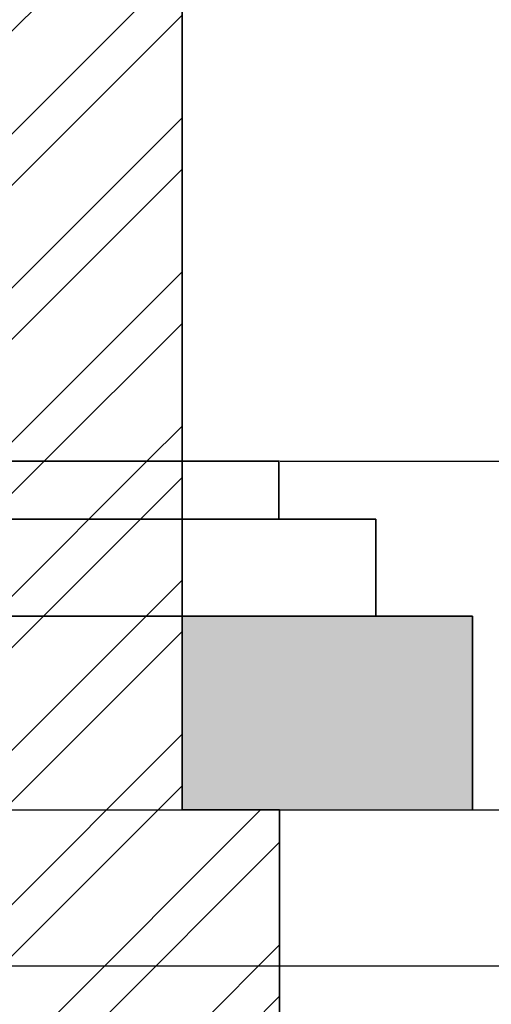
# Model space of a CAD drawing. Units: inches. Extents: x -301 to 715, y -607 to 364.
# Tile 35 of 141: x 135 to 159, y -492 to -441. Entities that reach past the tile are written whole.
import ezdxf

# ---------------------------------------------------------------- set-up
doc = ezdxf.new("R2010")
doc.units = ezdxf.units.IN
doc.header["$MEASUREMENT"] = 0
for name, color, linetype, lineweight in [('A-ANNO-DIMS', 2, 'Continuous', 18), ('A-GRND', 7, 'Continuous', 25), ('A-SECT', 1, 'Continuous', 35), ('A-SECT-PATT', 8, 'Continuous', 13), ('S-FNDN', 2, 'Continuous', 35)]:
    doc.layers.add(name, color=color, linetype=linetype, lineweight=lineweight)
doc.styles.get("Standard").update_dxf_attribs({"font": 'arial.ttf'})
doc.dimstyles.get("Standard").update_dxf_attribs({"dimtxt": 0.18, "dimasz": 0.18, "dimexe": 0.18, "dimexo": 0.0625, "dimgap": 0.09, "dimtad": 0, "dimtih": 1, "dimtoh": 1, "dimdec": 1, "dimzin": 0, "dimdsep": 46, "dimlunit": 4, "dimtxsty": 'Standard', "dimcen": 0.09, "dimclrd": 3, "dimclre": 4, "dimclrt": 6, "dimadec": 0, "dimazin": 0, "dimtfac": 1, "dimtdec": 1, "dimtofl": 0, "dimtmove": 0, "dimatfit": 3, "dimfxl": 1, "dimtfill": 2, "dimtfillclr": 51, "dimtolj": 1, "dimtzin": 0, "dimarcsym": 0})
pattern_1 = [(45, (10.321, 33.8764), (-3.977476, 3.977476), []), (45, (12.973, 33.8764), (-3.977476, 3.977476), [])]

# ---------------------------------------------------------------- blocks, each defined once
blk = doc.blocks.new('*D76')
at = {"layer": 'A-ANNO-DIMS', "color": 0, "lineweight": -2, "transparency": 16777216}
for p, q in [((158.28, -324.519), (162.311, -324.519)), ((162.131, -329.519), (162.131, -400.354)), ((162.131, -476.477), (162.131, -405.643)), ((158.28, -481.477), (162.311, -481.477))]:
    blk.add_line(p, q, dxfattribs=at)
at = {"layer": 'A-ANNO-DIMS', "color": 0, "transparency": 16777216}
for points in [[(161.297, -329.519), (162.964, -329.519), (162.131, -324.519)], [(161.297, -476.477), (162.964, -476.477), (162.131, -481.477)]]:
    blk.add_solid(points, dxfattribs=at)
at = {"layer": 'Defpoints', "color": 0, "transparency": 16777216}
for p in [(158.218, -324.519), (162.131, -324.519), (158.218, -481.477)]:
    blk.add_point(p, dxfattribs=at)
at = {"layer": 'A-ANNO-DIMS', "color": 0, "transparency": 16777216, "insert": (162.131, -402.998), "char_height": 5, "attachment_point": 5, "bg_fill": 1, "box_fill_scale": 1.25, "bg_fill_color": 51, "bg_fill_transparency": 0}
blk.add_mtext('\\A1;13\'-1"', dxfattribs=at)
blk = doc.blocks.new('*D80')
at = {"layer": 'A-ANNO-DIMS', "color": 0, "lineweight": -2, "transparency": 16777216}
for p, q in [((176.814, -481.477), (176.814, -476.477)), ((176.814, -476.477), (181.814, -476.477)), ((153.318, -481.477), (176.994, -481.477)), ((176.814, -488.477), (176.814, -486.477)), ((153.318, -493.477), (176.994, -493.477))]:
    blk.add_line(p, q, dxfattribs=at)
at = {"layer": 'A-ANNO-DIMS', "color": 0, "transparency": 16777216}
for points in [[(175.981, -486.477), (177.648, -486.477), (176.814, -481.477)], [(175.981, -488.477), (177.648, -488.477), (176.814, -493.477)]]:
    blk.add_solid(points, dxfattribs=at)
at = {"layer": 'Defpoints', "color": 0, "transparency": 16777216}
for p in [(153.255, -481.477), (176.814, -481.477), (153.255, -493.477)]:
    blk.add_point(p, dxfattribs=at)
at = {"layer": 'A-ANNO-DIMS', "color": 0, "transparency": 16777216, "insert": (183.969, -476.477), "char_height": 5, "attachment_point": 5, "bg_fill": 1, "box_fill_scale": 1.25, "bg_fill_color": 51, "bg_fill_transparency": 0}
blk.add_mtext("\\A1;1'", dxfattribs=at)
blk = doc.blocks.new('*D81')
at = {"layer": 'A-ANNO-DIMS', "color": 0, "lineweight": -2, "transparency": 16777216}
for p, q in [((155.28, -385.477), (177.024, -385.477)), ((176.844, -390.477), (176.844, -430.835)), ((176.844, -476.477), (176.844, -436.12)), ((158.28, -481.477), (177.024, -481.477))]:
    blk.add_line(p, q, dxfattribs=at)
at = {"layer": 'A-ANNO-DIMS', "color": 0, "transparency": 16777216}
for points in [[(176.011, -390.477), (177.678, -390.477), (176.844, -385.477)], [(176.011, -476.477), (177.678, -476.477), (176.844, -481.477)]]:
    blk.add_solid(points, dxfattribs=at)
at = {"layer": 'Defpoints', "color": 0, "transparency": 16777216}
for p in [(155.218, -385.477), (158.218, -481.477), (176.844, -481.477)]:
    blk.add_point(p, dxfattribs=at)
at = {"layer": 'A-ANNO-DIMS', "color": 0, "transparency": 16777216, "insert": (176.844, -433.477), "char_height": 5, "attachment_point": 5, "bg_fill": 1, "box_fill_scale": 1.25, "bg_fill_color": 51, "bg_fill_transparency": 0}
blk.add_mtext("\\A1;8'", dxfattribs=at)
blk = doc.blocks.new('*D176')
at = {"layer": 'A-ANNO-DIMS', "color": 4, "lineweight": -2, "transparency": 16777216}
for p, q in [((148.28, -324.477), (215.605, -324.477)), ((-15.22, -540.477), (215.605, -540.477))]:
    blk.add_line(p, q, dxfattribs=at)
at = {"layer": 'A-ANNO-DIMS', "color": 3, "lineweight": -2, "transparency": 16777216}
for p, q in [((215.425, -324.657), (215.425, -432.296)), ((215.425, -540.297), (215.425, -432.659))]:
    blk.add_line(p, q, dxfattribs=at)
at = {"layer": 'A-ANNO-DIMS', "color": 3, "transparency": 16777216}
for points in [[(215.395, -324.657), (215.455, -324.657), (215.425, -324.477)], [(215.395, -540.297), (215.455, -540.297), (215.425, -540.477)]]:
    blk.add_solid(points, dxfattribs=at)
at = {"layer": 'Defpoints', "color": 0, "transparency": 16777216}
for p in [(148.218, -324.477), (-15.282, -540.477), (215.425, -540.477)]:
    blk.add_point(p, dxfattribs=at)
at = {"layer": 'A-ANNO-DIMS', "color": 6, "transparency": 16777216, "insert": (215.425, -432.477), "char_height": 0.18, "attachment_point": 5, "bg_fill": 1, "box_fill_scale": 1.25, "bg_fill_color": 51, "bg_fill_transparency": 0}
blk.add_mtext('\\A1;18\'-0"', dxfattribs=at)
blk = doc.blocks.new('*D188')
at = {"layer": 'A-ANNO-DIMS', "color": 4, "lineweight": -2, "transparency": 16777216}
for p, q in [((148.28, -463.477), (215.605, -463.477)), ((158.28, -481.477), (215.605, -481.477))]:
    blk.add_line(p, q, dxfattribs=at)
at = {"layer": 'A-ANNO-DIMS', "color": 3, "lineweight": -2, "transparency": 16777216}
for p, q in [((215.425, -463.657), (215.425, -472.296)), ((215.425, -481.297), (215.425, -472.659))]:
    blk.add_line(p, q, dxfattribs=at)
at = {"layer": 'A-ANNO-DIMS', "color": 3, "transparency": 16777216}
for points in [[(215.395, -463.657), (215.455, -463.657), (215.425, -463.477)], [(215.395, -481.297), (215.455, -481.297), (215.425, -481.477)]]:
    blk.add_solid(points, dxfattribs=at)
at = {"layer": 'Defpoints', "color": 0, "transparency": 16777216}
for p in [(148.218, -463.477), (215.425, -463.477), (158.218, -481.477)]:
    blk.add_point(p, dxfattribs=at)
at = {"layer": 'A-ANNO-DIMS', "color": 6, "transparency": 16777216, "insert": (215.425, -472.477), "char_height": 0.18, "attachment_point": 5, "bg_fill": 1, "box_fill_scale": 1.25, "bg_fill_color": 51, "bg_fill_transparency": 0}
blk.add_mtext('\\A1;1\'-6"', dxfattribs=at)
blk = doc.blocks.new('*D200')
at = {"layer": 'A-ANNO-DIMS', "color": 4, "lineweight": -2, "transparency": 16777216}
for p, q in [((412.955, -393.552), (121.926, -393.552)), ((412.955, -489.552), (121.926, -489.552))]:
    blk.add_line(p, q, dxfattribs=at)
at = {"layer": 'A-ANNO-DIMS', "color": 3, "lineweight": -2, "transparency": 16777216}
for p, q in [((122.106, -393.732), (122.106, -441.371)), ((122.106, -489.372), (122.106, -441.734))]:
    blk.add_line(p, q, dxfattribs=at)
at = {"layer": 'A-ANNO-DIMS', "color": 3, "transparency": 16777216}
for points in [[(122.076, -393.732), (122.136, -393.732), (122.106, -393.552)], [(122.076, -489.372), (122.136, -489.372), (122.106, -489.552)]]:
    blk.add_solid(points, dxfattribs=at)
at = {"layer": 'Defpoints', "color": 0, "transparency": 16777216}
for p in [(122.106, -393.552), (413.018, -393.552), (413.018, -489.552)]:
    blk.add_point(p, dxfattribs=at)
at = {"layer": 'A-ANNO-DIMS', "color": 6, "transparency": 16777216, "insert": (122.106, -441.552), "char_height": 0.18, "attachment_point": 5, "bg_fill": 1, "box_fill_scale": 1.25, "bg_fill_color": 51, "bg_fill_transparency": 0}
blk.add_mtext('\\A1;8\'-0"', dxfattribs=at)

msp = doc.modelspace()

# ---------------------------------------------------------------- hatches: boundary and pattern name
at = {"layer": 'A-SECT-PATT'}
h = msp.add_hatch(dxfattribs=at)
h.set_pattern_fill('ANSI32', color=256, scale=15)
h.set_pattern_definition(pattern_1)
h.paths.add_polyline_path([(-185.282, -324.477), (-199.282, -324.477), (-199.282, -329.477), (-194.282, -329.477), (-194.282, -353.477), (-185.282, -353.477)])
h.paths.add_polyline_path([(-185.282, -361.477), (-193.904, -361.477), (-193.982, -377.537), (-185.282, -377.537)])
h.paths.add_polyline_path([(143.218, -329.477), (148.218, -329.477), (148.218, -324.477), (134.255, -324.477), (134.255, -353.477), (143.218, -353.477)])
h.paths.add_polyline_path([(143.218, -361.477), (134.255, -361.477), (134.255, -377.477), (143.218, -377.477)])
h.paths.add_polyline_path([(-185.282, -439.477), (-194.282, -439.477), (-194.282, -463.477), (-185.282, -463.477)])
h.paths.add_polyline_path([(-185.282, -471.477), (-194.282, -471.477), (-194.282, -481.477), (-185.282, -481.477)])
h.paths.add_polyline_path([(-185.282, -463.477), (-194.282, -463.477), (-194.282, -466.477), (-185.282, -466.477)])
h.paths.add_polyline_path([(-185.282, -466.477), (-194.282, -466.477), (-194.282, -471.477), (-185.282, -471.477)])
h.paths.add_polyline_path([(-180.282, -481.477), (-185.282, -481.477), (-194.282, -481.477), (-199.282, -481.477), (-199.282, -493.477), (-180.282, -493.477)])
h.paths.add_polyline_path([(-175.282, -493.477), (-180.282, -493.477), (-199.282, -493.477), (-204.282, -493.477), (-204.282, -511.477), (-175.282, -511.477)])
h.paths.add_polyline_path([(-170.282, -511.477), (-175.282, -511.477), (-204.282, -511.477), (-209.282, -511.477), (-209.282, -535.477), (-170.282, -535.477)])
h.paths.add_polyline_path([(-35.282, -463.477), (-41.282, -463.477), (-41.282, -466.477), (-35.282, -466.477)])
h.paths.add_polyline_path([(-35.282, -466.477), (-41.282, -466.477), (-41.282, -471.477), (-35.282, -471.477)])
h.paths.add_polyline_path([(-35.282, -471.477), (-41.282, -471.477), (-41.282, -481.477), (-35.282, -481.477)])
h.paths.add_polyline_path([(-30.282, -481.477), (-46.282, -481.477), (-46.282, -493.477), (-30.282, -493.477)])
h.paths.add_polyline_path([(-25.282, -493.477), (-30.282, -493.477), (-46.282, -493.477), (-51.282, -493.477), (-51.282, -511.477), (-25.282, -511.477)])
h.paths.add_polyline_path([(-20.282, -511.477), (-25.282, -511.477), (-51.282, -511.477), (-56.282, -511.477), (-56.282, -535.477), (-20.282, -535.477)])
h.paths.add_polyline_path([(143.218, -463.477), (134.255, -463.477), (134.255, -466.477), (143.218, -466.477)])
h.paths.add_polyline_path([(143.218, -466.477), (134.255, -466.477), (134.255, -471.477), (143.218, -471.477)])
h.paths.add_polyline_path([(143.218, -471.477), (134.255, -471.477), (134.255, -481.477), (143.218, -481.477)])
h.paths.add_polyline_path([(148.255, -481.477), (143.255, -481.477), (134.255, -481.477), (129.255, -481.477), (129.255, -493.477), (148.255, -493.477)])
h.paths.add_polyline_path([(153.255, -493.477), (148.255, -493.477), (129.255, -493.477), (124.255, -493.477), (124.255, -511.477), (153.255, -511.477)])
h.paths.add_polyline_path([(158.255, -511.477), (153.255, -511.477), (124.255, -511.477), (119.255, -511.477), (119.255, -535.477), (158.255, -535.477)])
h = msp.add_hatch(dxfattribs=at)
h.set_pattern_fill('AR-CONC', color=256, scale=0.5)
h.set_pattern_definition([(50, (10.3213, 33.8764), (3.586301, -0.31376), [0.375, -4.125]), (355, (10.3213, 33.8764), (-0.693757, 3.76096), [0.3, -3.3]), (100.45144, (10.62, 33.8502), (2.892544, 3.4472), [0.3187, -3.50571]), (46.1842, (10.3213, 34.8764), (5.336207, -0.827596), [0.5625, -6.1875]), (96.6356, (10.766, 34.8074), (4.67331, 4.870593), [0.47805, -5.25857]), (351.1842, (10.321, 34.8764), (4.67331, 4.870593), [0.45, -4.95]), (21, (10.8213, 34.6264), (2.984535, -2.013094), [0.375, -4.125]), (326, (10.8213, 34.6264), (1.216577, 3.62575), [0.3, -3.3]), (71.45144, (11.07, 34.4586), (4.201112, 1.612656), [0.3187, -3.50571]), (37.5, (10.3213, 33.8764), (0.0607993, 1.6644693), [0, -3.26, 0, -3.35, 0, -3.3125]), (7.5, (10.3213, 33.8764), (1.3153477, 1.9720586), [0, -1.91, 0, -3.185, 0, -1.2625]), (327.5, (9.2063, 33.8764), (2.6691122, -0.1127744), [0, -1.25, 0, -3.9, 0, -5.175]), (317.5, (8.7063, 33.8764), (2.915931, 0.500525), [0, -1.625, 0, -2.59, 0, -3.675])])
h.paths.add_polyline_path([(-56.282, -535.477), (-61.282, -535.477), (-61.282, -540.477), (-15.282, -540.477), (-15.282, -535.477), (-20.282, -535.477)])
h.paths.add_polyline_path([(119.255, -535.477), (114.255, -535.477), (114.255, -540.477), (163.255, -540.477), (163.255, -535.477), (158.255, -535.477)])
h.paths.add_polyline_path([(-206.282, -471.477), (-209.282, -471.477), (-209.282, -481.477), (-206.282, -481.477), (-194.282, -481.477), (-194.282, -471.477)])
h.paths.add_polyline_path([(-41.282, -481.477), (-41.282, -471.477), (-185.282, -471.477), (-185.282, -481.477), (-180.282, -481.477)])
h.paths.add_polyline_path([(134.255, -481.477), (134.255, -471.477), (-35.282, -471.477), (-35.282, -481.477), (-30.282, -481.477)])
h.paths.add_polyline_path([(155.218, -481.477), (158.218, -481.477), (158.218, -471.477), (153.218, -471.477), (143.218, -471.477), (143.218, -481.477), (148.255, -481.477)])
h.paths.add_polyline_path([(-193.88, -356.477), (-193.904, -361.477), (143.218, -361.477), (143.218, -356.477)])
h = msp.add_hatch(dxfattribs=at)
h.set_pattern_fill('ANSI32', color=256, scale=15)
h.set_pattern_definition(pattern_1)
h.paths.add_polyline_path([(-35.282, -361.477), (-41.282, -361.477), (-41.282, -376.452), (-35.282, -376.452)])
h.paths.add_polyline_path([(143.218, -439.477), (134.255, -439.477), (134.255, -463.477), (143.218, -463.477)])

# ---------------------------------------------------------------- linework, layer by layer
at = {"layer": 'A-GRND'}
for p, q in [((-206.282, -481.477), (155.218, -481.477)), ((155.218, -481.477), (191.218, -481.477))]:
    msp.add_line(p, q, dxfattribs=at)
at = {"layer": 'A-SECT'}
for p, q in [((143.218, -353.477), (143.218, -481.477)), ((-199.282, -463.477), (148.255, -463.477)), ((143.218, -463.477), (148.218, -463.477)), ((148.218, -463.477), (148.218, -466.477)), ((-204.282, -466.477), (153.218, -466.477)), ((148.218, -466.477), (153.218, -466.477)), ((153.218, -466.477), (153.218, -471.477)), ((-206.282, -471.477), (155.218, -471.477)), ((153.218, -471.477), (158.218, -471.477)), ((158.218, -471.477), (158.218, -481.477))]:
    msp.add_line(p, q, dxfattribs=at)
at = {"layer": 'S-FNDN'}
for p, q in [((143.255, -481.477), (148.255, -481.477)), ((148.255, -481.477), (148.255, -493.477))]:
    msp.add_line(p, q, dxfattribs=at)

# ---------------------------------------------------------------- dimensions: what is measured, and where the dimension line sits
at = {"layer": 'A-ANNO-DIMS'}
for base, p1, p2, override, picture, middle in [((215.425, -540.477), (148.218, -324.477), (-15.282, -540.477), {"dimdec": 1, "dimlfac": 1, "dimrnd": 0, "dimzin": 1, "dimdsep": 46, "dimlunit": 4, "dimfrac": 2}, '*D176', (215.425, -432.477)), ((162.131, -324.519), (158.218, -481.477), (158.218, -324.519), {"dimtxt": 5, "dimasz": 5, "dimclrd": 0, "dimclre": 0, "dimclrt": 0}, '*D76', (162.131, -402.998)), ((176.844, -481.477), (155.218, -385.477), (158.218, -481.477), {"dimtxt": 5, "dimasz": 5, "dimclrd": 0, "dimclre": 0, "dimclrt": 0}, '*D81', (176.844, -433.477)), ((122.106, -393.552), (413.018, -489.552), (413.018, -393.552), {"dimdec": 1, "dimlfac": 1, "dimrnd": 0, "dimzin": 1, "dimdsep": 46, "dimlunit": 4, "dimfrac": 2}, '*D200', (122.106, -441.552)), ((215.425, -463.477), (158.218, -481.477), (148.218, -463.477), {"dimdec": 1, "dimlfac": 1, "dimrnd": 0, "dimzin": 1, "dimdsep": 46, "dimlunit": 4, "dimfrac": 2}, '*D188', (215.425, -472.477)), ((176.814, -481.477), (153.255, -493.477), (153.255, -481.477), {"dimtxt": 5, "dimasz": 5, "dimclrd": 0, "dimclre": 0, "dimclrt": 0}, '*D80', (183.969, -476.477))]:
    dim = msp.add_linear_dim(base=base, p1=p1, p2=p2, angle=90, dimstyle='Standard', override=override, dxfattribs=at)
    dim.commit()
    dim.dimension.update_dxf_attribs({"geometry": picture, "text_midpoint": middle})

doc.saveas('drawing.dxf')
